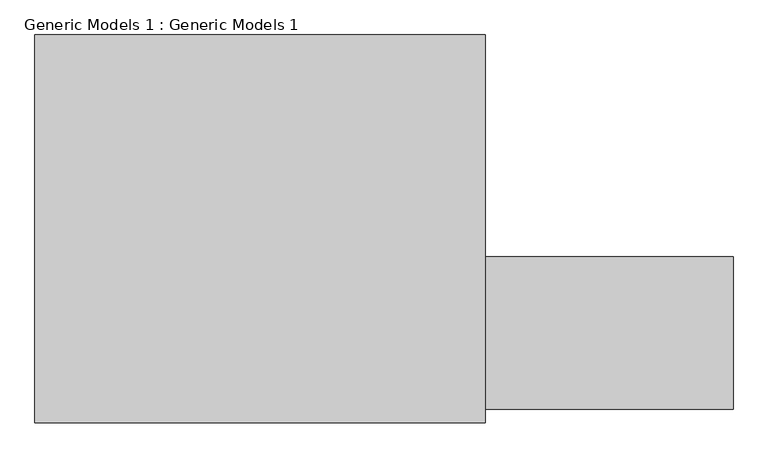
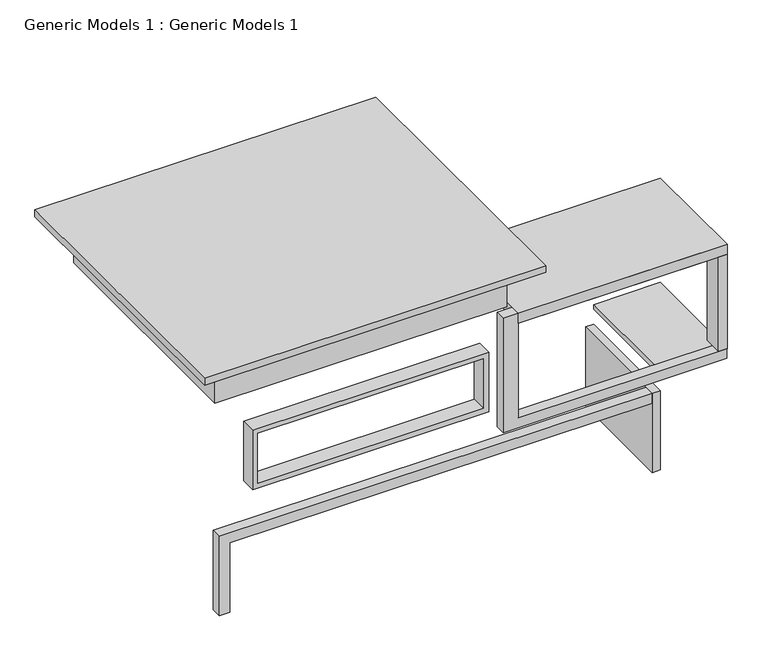
"""IFC4 building model written with IfcOpenShell, lengths in millimetres: proxy geometry, Generic Models 1 : Generic Models 1."""

from ifc_helpers import new_model, si_unit, frame, origin, origin_with_axes, place, context, project, spatial, polyline, outline, extrude, faceted_brep, source, transform, mapped, element, save


def generic_models_1_generic_models_1_da173db9(model_context):
    return source(origin(), model_context, "Body", "SolidModel", [
        faceted_brep([(1709.2319735, 9452.4286055, 7690.2776821), (-8196.7680265, 9452.4286055, 7690.2776821), (-8196.7680265, 918.0286055, 7690.2776821), (1709.2319735, 918.0286055, 7690.2776821), (1709.2319735, 9452.4286055, 7487.0776821), (1709.2319735, 918.0286055, 7487.0776821), (-8196.7680265, 918.0286055, 7487.0776821), (-8196.7680265, 9452.4286055, 7487.0776821), (1531.4319735, 9249.2286055, 7487.0776821), (-8044.3680265, 9249.2286055, 7487.0776821), (-8044.3680265, 1121.2286055, 7487.0776821), (1531.4319735, 1121.2286055, 7487.0776821), (1531.4319735, 9249.2286055, 7563.2776821), (1531.4319735, 1121.2286055, 7563.2776821), (-8044.3680265, 1121.2286055, 7563.2776821), (-8044.3680265, 9249.2286055, 7563.2776821)], [[[0, 1, 2, 3]], [[4, 5, 6, 7], [8, 9, 10, 11]], [[1, 0, 4, 7]], [[2, 1, 7, 6]], [[3, 2, 6, 5]], [[0, 3, 5, 4]], [[12, 13, 14, 15]], [[12, 15, 9, 8]], [[15, 14, 10, 9]], [[14, 13, 11, 10]], [[13, 12, 8, 11]]]),
        extrude(outline(polyline([(998.0319735, 1631.0040735), (-7485.5680265, 1631.0040735), (-7485.5680265, 8741.2286055), (998.0319735, 8741.2286055), (998.0319735, 1631.0040735)])), frame((0.0, 0.0, 6248.4), z_axis=(0.0, 0.0, 1.0), x_axis=(1.0, 0.0, 0.0)), (0.0, 0.0, 1.0), 1238.6776821),
        extrude(outline(polyline([(4985.8319735, 4575.6286055), (5214.4319735, 4575.6286055), (5214.4319735, 1224.6040735), (4985.8319735, 1224.6040735), (4985.8319735, 4575.6286055)])), origin_with_axes(), (0.0, 0.0, 1.0), 2438.4),
        extrude(outline(polyline([(2438.4, -7587.1680265), (0.0, -7587.1680265), (0.0, -7282.3680265), (2133.6, -7282.3680265), (2133.6, 4985.8319735), (2438.4, 4985.8319735), (2438.4, -7587.1680265)])), frame((0.0, 1224.6040735, 0.0), z_axis=(0.0, 1.0, 0.0), x_axis=(0.0, 0.0, 1.0)), (0.0, 0.0, 1.0), 304.8),
        extrude(outline(polyline([(1099.6319735, 4575.6286055), (7157.5319735, 4575.6286055), (7157.5319735, 1224.3818454), (1099.6319735, 1224.3818454), (1099.6319735, 4575.6286055)])), frame((0.0, 0.0, 5943.6), z_axis=(0.0, 0.0, 1.0), x_axis=(1.0, 0.0, 0.0)), (0.0, 0.0, 1.0), 304.8),
        extrude(outline(polyline([(7157.5319735, 1783.1818454), (7157.5319735, 1224.3818454), (6903.5319735, 1224.3818454), (6903.5319735, 1783.1818454), (7157.5319735, 1783.1818454)])), frame((0.0, 0.0, 3047.9793129), z_axis=(0.0, 0.0, 1.0), x_axis=(1.0, 0.0, 0.0)), (0.0, 0.0, 1.0), 2895.6206871),
        extrude(outline(polyline([(7157.5319735, 4575.6286055), (7157.5319735, 1529.4040735), (5214.4319735, 1529.4040735), (5214.4319735, 4575.6286055), (7157.5319735, 4575.6286055)])), frame((0.0, 0.0, 2895.5793129), z_axis=(0.0, 0.0, 1.0), x_axis=(1.0, 0.0, 0.0)), (0.0, 0.0, 1.0), 152.4),
        extrude(outline(polyline([(2743.2, 657.3620017), (2743.2, 7157.5319735), (3047.9793129, 7157.5319735), (3047.9793129, 1099.6319735), (5943.6, 1099.6319735), (5943.6, 6473.9721041), (6248.4, 6473.9721041), (6248.4, 657.3620017), (2743.2, 657.3620017)])), frame((0.0, 1224.6040735, 0.0), z_axis=(0.0, 1.0, 0.0), x_axis=(0.0, 0.0, 1.0)), (0.0, 0.0, 1.0), 304.8),
        extrude(outline(polyline([(5486.4, -6710.8680265), (3657.6, -6710.8680265), (3657.6, 147.1458376), (5486.4, 147.1458376), (5486.4, -6710.8680265)]), holes=[polyline([(5334.0, -6558.4680265), (5334.0, -5.2541624), (3810.0, -5.2541624), (3810.0, -6558.4680265), (5334.0, -6558.4680265)])]), frame((0.0, 1070.4286055, 0.0), z_axis=(0.0, 1.0, 0.0), x_axis=(0.0, 0.0, 1.0)), (0.0, 0.0, 1.0), 457.2),
    ])


if __name__ == "__main__":
    model = new_model("IFC4")
    model_context = context("Model", 3, world=origin())
    ifc_project = project(units=[si_unit("LENGTHUNIT", "METRE", prefix="MILLI")], contexts=[model_context])
    site = spatial("IfcSite", under=ifc_project)
    building = spatial("IfcBuilding", under=site)
    placement = place(None, origin())
    generic_models_1_generic_models_1_shape = generic_models_1_generic_models_1_da173db9(model_context)
    element("IfcBuildingElementProxy", 1, Name="Generic Models 1 : Generic Models 1", ObjectType="Generic Models 1 : Generic Models 1", at=placement, inside=building, context=model_context, shape_type="MappedRepresentation", body=[
        mapped(generic_models_1_generic_models_1_shape, transform((0.0, 0.0, 0.0), x_axis=(1.0, 0.0, 0.0), y_axis=(0.0, 1.0, 0.0), z_axis=(0.0, 0.0, 1.0))),
    ])
    save(model, "model.ifc")

# Revit data of these elements
# Element 1 (IfcBuildingElementProxy, "Generic Models 1 : Generic Models 1")
#   Materials on its faces: "Gypsum Wall Board", "extrusion", "tile"
# Materials
#   "Gypsum Wall Board": class "Generic", colour RGB 127 127 127, transparency 0, Description = "Gypsum Wall Board", Cost = 0
#   "extrusion": class "Generic", colour RGB 120 120 120, transparency 0, Cost = 0
#   "tile": class "Generic", colour RGB 120 120 120, transparency 0, Cost = 0
